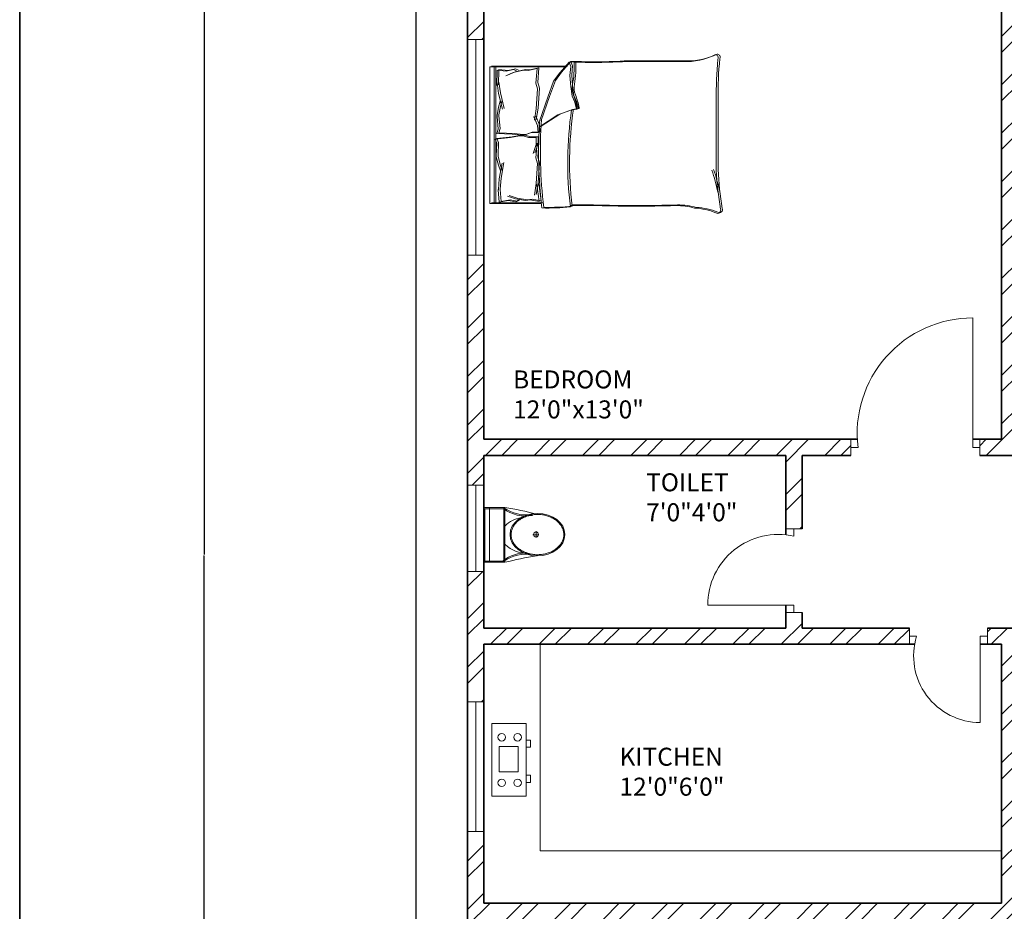
# Model space of a CAD drawing. Units: inches. Extents: x 1962 to 2771, y 1245 to 2660.
# Tile 85 of 114: x 1962 to 2236, y 2180 to 2428. Entities that reach past the tile are written whole.
import ezdxf

# ---------------------------------------------------------------- set-up
doc = ezdxf.new("R2010")
doc.units = ezdxf.units.IN
for name, color, linetype, lineweight in [('A-ANNO-DIMS', 2, 'Continuous', 18), ('A-ANNO-TTLB', 7, 'Continuous', 35), ('A-AREA-IDEN', 7, 'Continuous', 18), ('A-DOOR', 3, 'Continuous', 18), ('A-EQPM', 8, 'Continuous', 18), ('A-FLOR-CASE', 8, 'Continuous', 18), ('A-FLOR-FIXT', 8, 'Continuous', 18), ('A-FURN', 8, 'Continuous', 13), ('A-GLAZ', 4, 'Continuous', 18), ('A-WALL', 7, 'Continuous', 35), ('A-WALL-PATT', 252, 'Continuous', 13)]:
    doc.layers.add(name, color=color, linetype=linetype, lineweight=lineweight)
doc.styles.get("Standard").update_dxf_attribs({"font": 'arial.ttf'})
doc.dimstyles.get("Standard").update_dxf_attribs({"dimtxt": 0.18, "dimasz": 0.18, "dimexe": 0.18, "dimexo": 0.0625, "dimgap": 0.09, "dimtad": 0, "dimtih": 1, "dimtoh": 1, "dimdec": 4, "dimzin": 0, "dimdsep": 46, "dimtxsty": 'Standard', "dimcen": 0.09, "dimadec": 0, "dimazin": 0, "dimtfac": 1, "dimtdec": 4, "dimtofl": 0, "dimtmove": 0, "dimatfit": 3, "dimfxl": 1, "dimtolj": 1, "dimtzin": 0, "dimarcsym": 0})

# ---------------------------------------------------------------- blocks, each defined once
blk = doc.blocks.new('A$C31115884')
for p, q in [((283.1, 497.7), (223.4, 497.7)), ((257.5, 466.4), (257.5, 523.2)), ((0, 200), (0, 0)), ((520, 200), (0, 200)), ((10, 190), (10, 10)), ((510, 190), (10, 190)), ((510, 10), (510, 190)), ((520, 0), (520, 200)), ((510, 54.5), (0, 54.5)), ((10, 10), (510, 10)), ((0, 0), (520, 0))]:
    blk.add_line(p, q)
blk.add_circle((255.6, 496.4), 23.6)
for centre, radius, start, end in [((2777.7, -204.6), 2807, 165.4549, 171.71327), ((3237, 905), 2807, 188.28673, 194.5451), ((-294.5, 403.3), 364.7, 324.20913, 9.34987), ((-294.5, 403.3), 374.7, 324.20913, 9.34987), ((139.5, 406.2), 293.5, 315.84364, 2.65635), ((805.8, 403.3), 374.7, 179.20365, 215.79087), ((805.8, 403.3), 364.7, 170.65013, 215.79087), ((383.6, 406.2), 293.5, 190.27735, 224.15636)]:
    blk.add_arc(centre, radius, start, end)
blk.add_ellipse((256.2, 509.9), major_axis=(0, -260.7), ratio=0.772727)
blk.add_open_spline([(256.2, 259.2), (263.1, 259.2), (270, 259.7), (287.8, 262.3), (298.7, 265.1), (319.9, 273.1), (330.2, 278.4), (350.1, 291.1), (359.7, 298.7), (377.7, 315.9), (386.2, 325.5), (401.7, 346.6), (408.8, 358.1), (421.3, 382.5), (426.8, 395.5), (435.9, 422.4), (439.5, 436.4), (444.8, 465.1), (446.5, 479.7), (447.9, 509.2), (447.6, 524), (445, 553.3), (442.7, 567.8), (436.3, 596), (432.1, 609.7), (421.9, 636), (416, 648.6), (402.5, 672.1), (395, 683), (378.6, 703), (369.8, 712.1), (351.1, 728), (341.3, 734.8), (320.9, 746.2), (310.4, 750.7), (288.9, 757.3), (278, 759.4), (256, 761), (245, 760.6), (223.1, 757.2), (212.3, 754.3), (191.1, 746.1), (180.8, 740.7), (160.9, 727.8), (151.4, 720.1), (133.5, 702.7), (125.1, 693), (109.6, 671.7), (102.6, 660.2), (90.2, 635.7), (84.9, 622.7), (76, 595.6), (72.4, 581.6), (67.2, 552.9), (65.6, 538.2), (64.4, 508.8), (64.8, 494), (67.5, 464.7), (69.9, 450.2), (76.6, 422), (80.8, 408.3), (91.1, 382.2), (97.2, 369.7), (110.8, 346.3), (118.4, 335.4), (134.8, 315.6), (143.7, 306.7), (162.4, 290.9), (172.3, 284.2), (192.8, 273), (203.3, 268.6), (224.8, 262.2), (235.8, 260.2), (249.9, 259.3), (253, 259.2), (256.2, 259.2)], degree=3, knots=[0, 0, 0, 0, 0.110105, 0.110105, 0.285049, 0.285049, 0.459994, 0.459994, 0.634938, 0.634938, 0.809882, 0.809882, 0.984827, 0.984827, 1.159771, 1.159771, 1.334715, 1.334715, 1.50966, 1.50966, 1.684604, 1.684604, 1.859549, 1.859549, 2.034493, 2.034493, 2.209437, 2.209437, 2.384382, 2.384382, 2.559326, 2.559326, 2.73427, 2.73427, 2.909215, 2.909215, 3.084159, 3.084159, 3.259103, 3.259103, 3.434048, 3.434048, 3.608992, 3.608992, 3.783936, 3.783936, 3.958881, 3.958881, 4.133825, 4.133825, 4.30877, 4.30877, 4.483714, 4.483714, 4.658658, 4.658658, 4.833603, 4.833603, 5.008547, 5.008547, 5.183491, 5.183491, 5.358436, 5.358436, 5.53338, 5.53338, 5.708324, 5.708324, 5.883269, 5.883269, 6.058213, 6.058213, 6.233158, 6.233158, 6.283185, 6.283185, 6.283185, 6.283185])
blk = doc.blocks.new('BED-PLAN')
for p, q in [((22.05, 42.03), (19.47, 39.08)), ((22.05, 42.02), (19.47, 39.08)), ((22.56, 42.21), (19.98, 39.26)), ((22.56, 42.21), (19.98, 39.26)), ((23.44, 42.09), (22.05, 42.03, 3.08)), ((23.44, 42.09), (22.05, 42.02, 3.08)), ((22.55, 40.8), (22.05, 42.03)), ((22.55, 40.8), (22.05, 42.02)), ((23.95, 42.27), (22.56, 42.21, 3.08)), ((23.95, 42.27), (22.56, 42.21, 3.08)), ((23.06, 40.98), (22.56, 42.21)), ((23.06, 40.98), (22.56, 42.21)), ((0, 40.75), (21.15, 40.75)), ((0, 40.75), (21.15, 40.75)), ((0, 2.76), (0, 40.75)), ((0.51, 40.93), (21.66, 40.93)), ((0.51, 40.93), (21.66, 40.93)), ((1.22, 2.76), (1.22, 40.75)), ((1.22, 2.76), (1.22, 40.75)), ((1.73, 2.95), (1.73, 40.93)), ((1.73, 2.95), (1.73, 40.93)), ((2.03, 39.83), (1.96, 35.54)), ((2.03, 39.83), (1.96, 35.54)), ((2.03, 39.83), (4.58, 39.53)), ((2.03, 39.83), (4.58, 39.53)), ((2.54, 40.02), (2.46, 35.72)), ((2.54, 40.02), (2.46, 35.72)), ((2.54, 40.02), (5.09, 39.72)), ((2.54, 40.02), (5.09, 39.72)), ((6.56, 39.2), (4.43, 38.26)), ((6.56, 39.2), (4.43, 38.26)), ((4.58, 39.53), (6.63, 40.01)), ((4.58, 39.53), (6.63, 40.01)), ((7.07, 39.38), (4.94, 38.44)), ((7.07, 39.38), (4.94, 38.44)), ((5.09, 39.72), (7.14, 40.19)), ((5.09, 39.72), (7.14, 40.19)), ((9.4, 39.83), (6.56, 39.2)), ((9.4, 39.83), (6.56, 39.2)), ((6.63, 40.01), (7.46, 39.6)), ((6.63, 40.01), (7.46, 39.6)), ((9.91, 40.02), (7.07, 39.38)), ((9.91, 40.02), (7.07, 39.38)), ((7.14, 40.19), (7.97, 39.78)), ((7.14, 40.19), (7.97, 39.78)), ((10.68, 39.68), (9.4, 39.83)), ((10.68, 39.68), (9.4, 39.83)), ((11.19, 39.87), (9.91, 40.02)), ((11.19, 39.87), (9.91, 40.02)), ((13.17, 40.3), (10.68, 39.68)), ((13.17, 40.3), (10.68, 39.68)), ((13.68, 40.48), (11.19, 39.87)), ((13.68, 40.48), (11.19, 39.87)), ((12.85, 36.22), (13.17, 40.3)), ((12.85, 36.22), (13.17, 40.3)), ((13.36, 36.4), (13.68, 40.48)), ((13.36, 36.4), (13.68, 40.48)), ((19.47, 39.08), (17.75, 36.74)), ((19.47, 39.08), (17.75, 36.74)), ((19.98, 39.26), (18.26, 36.92)), ((19.98, 39.26), (18.26, 36.92)), ((22.3, 38.34), (22.55, 40.8)), ((22.3, 38.34), (22.55, 40.8)), ((22.55, 35.26), (22.3, 38.34)), ((22.55, 35.26), (22.3, 38.34)), ((22.81, 38.52), (23.06, 40.98)), ((22.81, 38.52), (23.06, 40.98)), ((23.06, 35.45), (22.81, 38.52)), ((23.06, 35.44), (22.81, 38.52)), ((1.96, 35.54), (2.02, 36.34)), ((1.96, 35.54), (2.02, 36.34)), ((2.02, 36.34), (2.44, 33.32)), ((2.02, 36.34), (2.44, 33.32)), ((2.46, 35.72), (2.53, 36.52)), ((2.46, 35.72), (2.53, 36.52)), ((2.53, 36.52), (2.95, 33.5)), ((2.53, 36.52), (2.95, 33.5)), ((13.3, 34.66), (12.85, 36.22)), ((13.3, 34.66), (12.85, 36.22)), ((13.8, 34.84), (13.36, 36.4)), ((13.8, 34.84), (13.36, 36.4)), ((17.75, 36.74), (16.15, 32.31)), ((17.75, 36.74), (16.15, 32.31)), ((18.26, 36.92), (16.66, 32.49)), ((18.26, 36.92), (16.66, 32.49)), ((2.44, 33.32), (3.52, 29.01)), ((2.44, 33.32), (3.52, 29.01)), ((2.95, 33.5), (4.02, 29.19)), ((2.95, 33.5), (4.02, 29.19)), ((12.95, 29.09), (13.3, 34.66)), ((12.95, 29.09), (13.3, 34.66)), ((13.46, 29.27), (13.8, 34.84)), ((13.46, 29.27), (13.8, 34.84)), ((22.92, 32.56), (22.55, 35.26)), ((22.92, 32.55), (22.55, 35.26)), ((23.42, 32.74), (23.06, 35.45)), ((23.42, 32.74), (23.06, 35.44)), ((2.92, 31.16), (2.45, 29.52)), ((2.92, 31.16), (2.45, 29.52)), ((3.43, 31.34), (2.96, 29.7)), ((3.43, 31.34), (2.96, 29.7)), ((16.15, 32.31), (13.82, 25.68)), ((16.15, 32.31), (13.82, 25.68)), ((16.66, 32.49), (14.33, 25.86)), ((16.66, 32.49), (14.33, 25.86)), ((23.65, 30.95), (22.92, 32.56)), ((23.65, 30.95), (22.92, 32.55)), ((24.16, 31.14), (23.42, 32.74)), ((24.16, 31.14), (23.42, 32.74)), ((24.15, 28.99), (23.65, 30.95)), ((24.15, 28.98), (23.65, 30.95)), ((24.65, 29.17), (24.16, 31.14)), ((24.65, 29.17), (24.16, 31.14)), ((62.99, 11.98), (62.99, 31.54)), ((62.99, 11.97), (62.99, 31.54)), ((63.5, 12.16), (63.5, 31.72)), ((63.5, 12.16), (63.5, 31.72)), ((2.45, 29.52), (2.02, 27.19)), ((2.45, 29.52), (2.02, 27.19)), ((2.96, 29.7), (2.52, 27.37)), ((2.96, 29.7), (2.52, 27.37)), ((12.42, 25.89), (12.95, 29.09)), ((12.42, 25.89), (12.95, 29.09)), ((12.93, 26.07), (13.46, 29.27)), ((12.93, 26.07), (13.46, 29.27)), ((13.82, 24.05), (18.98, 27.38)), ((13.82, 24.05), (18.98, 27.38)), ((14.33, 24.24), (19.49, 27.57)), ((14.33, 24.24), (19.49, 27.57)), ((18.98, 27.38), (22.55, 28.74)), ((18.98, 27.38), (22.55, 28.74)), ((19.49, 27.57), (23.06, 28.92)), ((19.49, 27.57), (23.06, 28.92)), ((22.55, 28.74), (24.15, 28.99)), ((22.55, 28.74), (24.15, 28.98)), ((23.06, 28.92), (24.65, 29.17)), ((23.06, 28.92), (24.65, 29.17)), ((2.02, 27.19), (2.03, 26.94)), ((2.02, 27.19), (2.03, 26.93)), ((2.03, 26.94), (2.37, 23.42)), ((2.03, 26.93), (2.37, 23.42)), ((2.52, 27.37), (2.54, 27.12)), ((2.52, 27.37), (2.54, 27.12)), ((2.54, 27.12), (2.88, 23.6)), ((2.54, 27.12), (2.88, 23.6)), ((13.31, 24.44), (12.28, 26.89)), ((13.31, 24.44), (12.28, 26.88)), ((13.81, 24.63), (12.79, 27.07)), ((13.81, 24.63), (12.79, 27.07)), ((2.37, 23.42), (1.98, 22.24)), ((2.37, 23.42), (1.98, 22.24)), ((1.98, 22.24), (6.25, 22.05)), ((1.98, 22.24), (6.25, 22.05)), ((2.88, 23.6), (2.49, 22.42)), ((2.88, 23.6), (2.49, 22.42)), ((2.49, 22.42), (6.76, 22.23)), ((2.49, 22.42), (6.76, 22.23)), ((6.25, 22.05), (8.81, 21.75)), ((6.25, 22.05), (8.81, 21.75)), ((6.76, 22.23), (9.31, 21.93)), ((6.76, 22.23), (9.31, 21.93)), ((9.31, 21.93), (10.35, 21.99)), ((9.31, 21.93), (10.35, 21.99)), ((9.84, 21.81), (11.3, 22.36)), ((9.84, 21.81), (11.3, 22.36)), ((10.35, 21.99), (11.81, 22.54)), ((10.35, 21.99), (11.81, 22.54)), ((11.3, 22.36), (13.43, 22.49)), ((11.3, 22.36), (13.43, 22.49)), ((11.81, 22.54), (13.94, 22.68)), ((11.81, 22.54), (13.94, 22.68)), ((13.43, 22.49), (13.31, 24.44)), ((13.43, 22.49), (13.31, 24.44)), ((13.94, 22.68), (13.81, 24.63)), ((13.94, 22.68), (13.81, 24.63)), ((1.49, 20.65), (5.74, 21.11)), ((1.49, 20.65), (5.74, 21.11)), ((1.95, 19.51), (1.49, 20.65)), ((1.95, 19.51), (1.49, 20.65)), ((1.83, 15.97), (1.95, 19.51)), ((1.83, 15.97), (1.95, 19.51)), ((1.99, 20.84), (6.25, 21.3)), ((1.99, 20.84), (6.25, 21.3)), ((2.45, 19.69), (1.99, 20.84)), ((2.45, 19.69), (1.99, 20.84)), ((2.34, 16.15), (2.45, 19.69)), ((2.34, 16.15), (2.45, 19.69)), ((5.74, 21.11), (8.27, 21.57)), ((5.74, 21.11), (8.27, 21.57)), ((6.25, 21.3), (8.78, 21.76)), ((6.25, 21.3), (8.78, 21.76)), ((8.27, 21.57), (9.3, 21.57)), ((8.27, 21.57), (9.3, 21.57)), ((8.78, 21.76), (9.81, 21.76)), ((8.78, 21.76), (9.81, 21.76)), ((8.81, 21.75), (9.84, 21.81)), ((8.81, 21.75), (9.84, 21.81)), ((9.3, 21.57), (10.8, 21.11)), ((9.3, 21.57), (10.8, 21.11)), ((9.81, 21.76), (11.3, 21.3)), ((9.81, 21.76), (11.3, 21.3)), ((10.8, 21.11), (12.93, 21.11)), ((10.8, 21.11), (12.93, 21.11)), ((11.3, 21.3), (13.44, 21.3)), ((11.3, 21.3), (13.44, 21.3)), ((13.44, 19.34), (12.57, 16.84)), ((13.44, 19.34), (12.57, 16.84)), ((12.85, 15.41), (13.17, 19.49)), ((12.85, 15.41), (13.17, 19.49)), ((12.93, 21.11), (12.93, 19.16)), ((12.93, 21.11), (12.93, 19.16)), ((13.36, 15.59), (13.68, 19.67)), ((13.36, 15.59), (13.68, 19.67)), ((13.44, 21.3), (13.44, 19.34)), ((13.44, 21.3), (13.44, 19.34)), ((12.93, 19.16), (12.06, 16.66)), ((12.93, 19.16), (12.06, 16.66)), ((1.83, 15.72), (1.83, 15.97)), ((1.83, 15.72), (1.83, 15.97)), ((2.41, 13.42), (1.83, 15.72)), ((2.41, 13.42), (1.83, 15.72)), ((2.34, 15.9), (2.34, 16.15)), ((2.34, 15.9), (2.34, 16.15)), ((2.91, 13.6), (2.34, 15.9)), ((2.91, 13.6), (2.34, 15.9)), ((2.64, 9.63), (3.44, 13.99)), ((2.64, 9.63), (3.44, 13.99)), ((3.14, 9.81), (3.95, 14.17)), ((3.14, 9.81), (3.95, 14.17)), ((13.3, 13.85), (12.85, 15.41)), ((13.3, 13.85), (12.85, 15.41)), ((12.95, 8.28), (13.3, 13.85)), ((12.95, 8.28), (13.3, 13.85)), ((13.8, 14.03), (13.36, 15.59)), ((13.8, 14.03), (13.36, 15.59)), ((13.46, 8.46), (13.8, 14.03)), ((13.46, 8.46), (13.8, 14.03)), ((2.98, 11.81), (2.41, 13.42)), ((2.98, 11.81), (2.41, 13.42)), ((3.49, 11.99), (2.91, 13.6)), ((3.49, 11.99), (2.91, 13.6)), ((2.41, 6.59), (2.64, 9.63)), ((2.41, 6.59), (2.64, 9.63)), ((2.91, 6.77), (3.14, 9.81)), ((2.91, 6.77), (3.14, 9.81)), ((12.42, 5.07), (12.95, 8.28)), ((12.42, 5.07), (12.95, 8.28)), ((12.93, 5.26), (13.46, 8.46)), ((12.93, 5.26), (13.46, 8.46)), ((12.95, 8.28), (13.21, 7.38)), ((12.95, 8.28), (13.21, 7.38)), ((13.46, 8.46), (13.72, 7.56)), ((13.46, 8.46), (13.72, 7.56)), ((2.39, 6.5), (2.41, 6.59)), ((2.39, 6.5), (2.41, 6.59)), ((2.65, 3.1), (2.39, 6.5)), ((2.65, 3.1), (2.39, 6.5)), ((2.9, 6.68), (2.91, 6.77)), ((2.9, 6.68), (2.91, 6.77)), ((3.16, 3.28), (2.9, 6.68)), ((3.16, 3.28), (2.9, 6.68)), ((13.21, 7.38), (13.78, 3.33)), ((13.21, 7.38), (13.78, 3.33)), ((13.72, 7.56), (14.29, 3.51)), ((13.72, 7.56), (14.29, 3.51)), ((14.4, 2.76), (0, 2.76)), ((14.4, 2.76), (0, 2.76)), ((14.9, 2.95), (0.51, 2.95)), ((14.9, 2.95), (0.51, 2.95)), ((2.64, 3.1), (5.16, 3.56)), ((2.64, 3.1), (5.16, 3.56)), ((3.14, 3.28), (5.67, 3.74)), ((3.14, 3.28), (5.67, 3.74)), ((7.12, 4.02), (4.93, 4.82)), ((7.12, 4.02), (4.93, 4.82)), ((5.16, 3.56), (7.23, 3.21)), ((5.16, 3.56), (7.23, 3.21)), ((7.63, 4.2), (5.44, 5)), ((7.63, 4.2), (5.44, 5)), ((5.67, 3.74), (7.74, 3.39)), ((5.67, 3.74), (7.74, 3.39)), ((9.99, 3.56), (7.12, 4.02)), ((9.99, 3.56), (7.12, 4.02)), ((7.23, 3.21), (8.04, 3.67)), ((7.23, 3.21), (8.04, 3.67)), ((10.5, 3.74), (7.63, 4.2)), ((10.5, 3.74), (7.63, 4.2)), ((7.74, 3.39), (8.55, 3.85)), ((7.74, 3.39), (8.55, 3.85)), ((11.26, 3.79), (9.99, 3.56)), ((11.26, 3.79), (9.99, 3.56)), ((11.76, 3.97), (10.5, 3.74)), ((11.76, 3.97), (10.5, 3.74)), ((13.78, 3.33), (11.26, 3.79)), ((13.78, 3.33), (11.26, 3.79)), ((14.29, 3.51), (11.76, 3.97)), ((14.29, 3.51), (11.76, 3.97))]:
    blk.add_line(p, q)
for centre, radius, start, end in [((54.58, 60.54), 18.33, 267.4714, 296.4681), ((54.58, 60.54), 18.33, 267.4714, 296.4681), ((55.09, 60.72), 18.33, 267.4714, 296.4681), ((55.09, 60.72), 18.33, 267.4714, 296.4681), ((62.69, 43.25), 0.876, 332.6588, 86.02), ((62.69, 43.25), 0.876, 332.6588, 86.02), ((63.2, 43.43), 0.876, 332.6588, 86.02), ((63.2, 43.43), 0.876, 332.6588, 86.02), ((-5.29, 40.8), 28.76, 349.8763, 2.5657), ((-5.29, 40.8), 28.76, 349.8763, 2.5657), ((28.87, 144.88), 102.94, 266.9791, 273.8365), ((28.87, 144.88), 102.94, 266.9791, 273.8365), ((-4.78, 40.98), 28.76, 349.8763, 2.5657), ((-4.78, 40.98), 28.76, 349.8763, 2.5657), ((29.37, 145.06), 102.94, 266.9791, 273.8365), ((29.37, 145.06), 102.94, 266.9791, 273.8365), ((53.91, -3583.94), 3626.16, 90.00217, 90.28689), ((53.91, -3583.94), 3626.16, 90.00217, 90.28689), ((54.42, -3583.75), 3626.16, 90.00217, 90.28689), ((54.42, -3583.75), 3626.16, 90.00217, 90.28689), ((168.74, 32.71), 105.75, 174.4998, 180.6351), ((168.74, 32.71), 105.75, 174.4998, 180.6351), ((169.24, 32.89), 105.75, 174.4998, 180.6351), ((169.24, 32.89), 105.75, 174.4998, 180.6351), ((27.87, 34.77), 4.95, 168.6608, 203.7384), ((27.87, 34.77), 4.95, 168.6608, 203.7384), ((28.38, 34.95), 4.95, 168.6608, 203.7384), ((28.38, 34.95), 4.95, 168.6608, 203.7384), ((1.69, 24.95), 23.57, 10.6617, 19.8806), ((1.69, 24.95), 23.57, 10.6617, 19.8806), ((1.18, 24.77), 23.57, 10.6617, 19.8806), ((1.18, 24.76), 23.57, 10.6617, 19.8806), ((124.25, 14.12), 102.56, 171.7845, 186.9006), ((124.25, 14.11), 102.56, 171.7845, 186.9006), ((124.76, 14.3), 102.56, 171.7845, 186.9006), ((124.76, 14.3), 102.56, 171.7845, 186.9006), ((24.2, 29.12), 0.147, 250.2464, 1.1377), ((24.2, 29.12), 0.147, 250.2464, 1.1377), ((24.7, 29.3), 0.147, 250.2464, 1.1377), ((24.7, 29.3), 0.147, 250.2464, 1.1377), ((144.71, 16.98), 131.13, 176.0865, 186.7821), ((144.71, 16.98), 131.13, 176.0865, 186.7821), ((145.22, 17.16), 131.13, 176.0865, 186.7821), ((145.22, 17.16), 131.13, 176.0865, 186.7821), ((-18.85, -13.69), 84.62, 13.3832, 17.7053), ((-18.85, -13.69), 84.62, 13.3832, 17.7053), ((-18.34, -13.51), 84.62, 13.3832, 17.7053), ((-18.34, -13.51), 84.62, 13.3832, 17.7053), ((159.64, 17.03), 96.78, 182.9958, 189.4091), ((159.64, 17.03), 96.78, 182.9958, 189.4091), ((160.15, 17.21), 96.78, 182.9958, 189.4091), ((160.15, 17.21), 96.78, 182.9958, 189.4091), ((15.97, 67.7), 66.22, 268.7218, 275.604), ((15.97, 67.7), 66.22, 268.7218, 275.604), ((16.48, 67.88), 66.22, 268.7218, 275.604), ((16.48, 67.88), 66.22, 268.7218, 275.604), ((24.78, -132.99), 135.22, 88.4762, 91.0082), ((24.78, -132.99), 135.22, 88.4762, 91.0082), ((25.29, -132.81), 135.22, 88.4762, 91.0082), ((25.29, -132.81), 135.22, 88.4762, 91.0082), ((40.23, 385.38), 383.38, 268.2277, 271.7185), ((40.23, 385.38), 383.38, 268.2277, 271.7185), ((40.74, 385.56), 383.38, 268.2277, 271.7185), ((40.74, 385.56), 383.38, 268.2277, 271.7185), ((51.28, -21.38), 23.56, 76.0648, 88.9113), ((51.28, -21.38), 23.56, 76.0648, 88.9113), ((51.79, -21.2), 23.56, 76.0648, 88.9113), ((51.79, -21.2), 23.56, 76.0648, 88.9113), ((55.86, -17.22), 18.73, 67.9751, 86.652), ((55.86, -17.22), 18.73, 67.9751, 86.652), ((56.37, -17.03), 18.73, 67.9751, 86.652), ((56.37, -17.03), 18.73, 67.9751, 86.652), ((63.37, 0.87), 0.866, 236.1736, 23.4781), ((63.37, 0.87), 0.866, 236.1736, 23.4781), ((63.87, 1.05), 0.866, 236.1736, 23.4781), ((63.87, 1.05), 0.866, 236.1736, 23.4781)]:
    blk.add_arc(centre, radius, start, end)
blk = doc.blocks.new('COOKTOP-4-BURNER')
for points in [[(0, 20.18), (9.48, 20.18), (9.48, 0), (0, 0)], [(2, 13.79), (7.26, 13.79), (7.26, 6.73), (2, 6.73)], [(9.48, 15.59), (10.71, 15.59), (10.71, 13.59), (9.48, 13.59)], [(9.48, 5.81), (10.71, 5.81), (10.71, 3.8), (9.48, 3.8)]]:
    blk.add_lwpolyline(points, close=True)
for centre in [(2.74, 16.38), (7.14, 16.38), (2.74, 3.71), (7.14, 3.71)]:
    blk.add_circle(centre, 1.05)
blk = doc.blocks.new('WIN-24IN-A')
for p, q in [((0, 24), (4.5, 24)), ((4.5, 24), (2.25, 24)), ((2.25, 24), (2.25, 0)), ((2.25, 0), (0, 0)), ((0, 0), (4.5, 0))]:
    blk.add_line(p, q)
blk = doc.blocks.new('WIN-60IN-A')
for p, q in [((0, 60), (4.5, 60)), ((4.5, 60), (2.25, 60)), ((2.25, 60), (2.25, 0)), ((2.25, 0), (0, 0)), ((0, 0), (4.5, 0))]:
    blk.add_line(p, q)
blk = doc.blocks.new('WIN-36IN-A')
for p, q in [((4.5, 36), (0, 36)), ((0, 36), (2.25, 36)), ((2.25, 36), (2.25, 0)), ((2.25, 0), (0, 0)), ((0, 0), (4.5, 0))]:
    blk.add_line(p, q)
blk = doc.blocks.new('*D40')
at = {"layer": 'A-ANNO-DIMS', "color": 0, "lineweight": -2, "transparency": 16777216}
for p, q in [((2072.02, 2033.91), (2072.02, 2583.47)), ((2072.2, 2583.29), (2366.02, 2583.29)), ((2660.63, 2583.29), (2366.81, 2583.29)), ((2660.81, 2524.41), (2660.81, 2583.47))]:
    blk.add_line(p, q, dxfattribs=at)
at = {"layer": 'A-ANNO-DIMS', "color": 0, "transparency": 16777216}
for points in [[(2072.2, 2583.32), (2072.2, 2583.26), (2072.02, 2583.29)], [(2660.63, 2583.32), (2660.63, 2583.26), (2660.81, 2583.29)]]:
    blk.add_solid(points, dxfattribs=at)
at = {"layer": 'Defpoints', "color": 0, "transparency": 16777216}
for p in [(2660.81, 2583.29), (2660.81, 2524.34), (2072.02, 2033.84)]:
    blk.add_point(p, dxfattribs=at)
at = {"layer": 'A-ANNO-DIMS', "color": 0, "transparency": 16777216, "insert": (2366.41, 2583.29), "char_height": 0.18, "attachment_point": 5}
blk.add_mtext('\\A1;588.8', dxfattribs=at)
blk = doc.blocks.new('*D43')
at = {"layer": 'A-ANNO-DIMS', "color": 0, "lineweight": -2, "transparency": 16777216}
for p, q in [((2086.24, 2524.34), (2012.89, 2524.34)), ((2013.07, 2524.16), (2013.07, 2279.28)), ((2013.07, 2034.02), (2013.07, 2278.91)), ((2071.96, 2033.84), (2012.89, 2033.84))]:
    blk.add_line(p, q, dxfattribs=at)
at = {"layer": 'A-ANNO-DIMS', "color": 0, "transparency": 16777216}
for points in [[(2013.04, 2524.16), (2013.1, 2524.16), (2013.07, 2524.34)], [(2013.04, 2034.02), (2013.1, 2034.02), (2013.07, 2033.84)]]:
    blk.add_solid(points, dxfattribs=at)
at = {"layer": 'Defpoints', "color": 0, "transparency": 16777216}
for p in [(2086.31, 2524.34), (2013.07, 2033.84), (2072.02, 2033.84)]:
    blk.add_point(p, dxfattribs=at)
at = {"layer": 'A-ANNO-DIMS', "color": 0, "transparency": 16777216, "insert": (2013.07, 2279.09), "char_height": 0.18, "attachment_point": 5}
blk.add_mtext('\\A1;490.5', dxfattribs=at)

msp = doc.modelspace()

# ---------------------------------------------------------------- hatches: boundary and pattern name
at = {"layer": 'A-WALL-PATT'}
h = msp.add_hatch(dxfattribs=at)
h.set_pattern_fill('ANSI32', color=256)
h.paths.add_polyline_path([(2090.8074, 2467.3437), (2141.6481, 2467.3437), (2141.6481, 2469.5937), (2141.6481, 2471.8437), (2086.3074, 2471.8437), (2086.3074, 2422.5333), (2090.8074, 2422.5333)])
h.paths.add_polyline_path([(2282.7664, 2471.8437), (2204.8982, 2471.8437), (2204.8982, 2467.3437), (2234.8074, 2467.3437), (2234.8074, 2311.3437), (2228.7492, 2311.3437), (2228.7492, 2306.8437), (2234.8074, 2306.8437), (2331.9227, 2306.8437), (2331.9227, 2309.0937), (2331.9227, 2311.3437), (2239.3074, 2311.3437), (2239.3074, 2467.3437), (2282.7664, 2467.3437), (2282.7664, 2469.5937)])
h.paths.add_polyline_path([(2471.4531, 2519.8437), (2552.011, 2519.8437), (2564.3996, 2519.8437), (2564.3996, 2511.1389), (2568.8996, 2511.1389), (2568.8996, 2524.3437), (2466.9531, 2524.3437), (2466.9531, 2471.8437), (2450.0749, 2471.8437), (2446.4672, 2471.8437), (2446.4672, 2467.3437), (2450.0749, 2467.3437), (2475.9988, 2467.3437), (2475.9988, 2469.5937), (2475.9988, 2471.8437), (2471.4531, 2471.8437)])
h.paths.add_polyline_path([(2575.2231, 2469.5937), (2575.2231, 2471.8437), (2568.8996, 2471.8437), (2568.8996, 2487.1389), (2564.3996, 2487.1389), (2564.3996, 2471.8437), (2556.511, 2471.8437), (2499.2904, 2471.8437), (2499.2904, 2467.3437), (2507.8074, 2467.3437), (2507.8074, 2311.3437), (2414.863, 2311.3437), (2414.863, 2306.8437), (2512.3074, 2306.8437), (2517.0114, 2306.8437), (2517.0114, 2309.0937), (2517.0114, 2311.3437), (2512.3074, 2311.3437), (2512.3074, 2467.3437), (2575.2231, 2467.3437)])
h.paths.add_polyline_path([(2660.8074, 2471.8437), (2600.9602, 2471.8437), (2600.9602, 2467.3437), (2656.3074, 2467.3437), (2656.3074, 2432.5704), (2660.8074, 2432.5704)])
h.paths.add_polyline_path([(2660.8074, 2372.5704), (2656.3074, 2372.5704), (2656.3074, 2311.3437), (2600.276, 2311.3437), (2600.276, 2309.0937), (2600.276, 2306.8437), (2656.3074, 2306.8437), (2656.3074, 2296.2593), (2660.8074, 2296.2593)])
h.paths.add_polyline_path([(2572.3074, 2306.8437), (2577.1385, 2306.8437), (2577.1385, 2311.3437), (2551.082, 2311.3437), (2551.082, 2306.8437), (2567.8074, 2306.8437), (2567.8074, 2258.8437), (2540.0574, 2258.8437), (2540.0574, 2256.5937), (2540.0574, 2254.3437), (2567.8074, 2254.3437), (2656.3074, 2254.3437), (2656.3074, 2236.9085), (2660.8074, 2236.9085), (2660.8074, 2272.2593), (2656.3074, 2272.2593), (2656.3074, 2258.8437), (2572.3074, 2258.8437)])
h.paths.add_polyline_path([(2512.3074, 2254.3437), (2518.8716, 2254.3437), (2518.8716, 2256.5937), (2518.8716, 2258.8437), (2507.8074, 2258.8437), (2507.8074, 2177.8437), (2567.8074, 2177.8437), (2567.8074, 2172.9628), (2572.3074, 2172.9628), (2572.3074, 2177.8437), (2656.3074, 2177.8437), (2656.3074, 2166.4846), (2660.8074, 2166.4846), (2660.8074, 2200.9085), (2656.3074, 2200.9085), (2656.3074, 2182.3437), (2512.3074, 2182.3437)])
h.paths.add_polyline_path([(2656.3074, 2129.8437), (2572.3074, 2129.8437), (2572.3074, 2150.3044), (2570.0574, 2150.3044), (2567.8074, 2150.3044), (2567.8074, 2129.8437), (2507.8074, 2129.8437), (2507.8074, 2116.3027), (2510.0574, 2116.3027), (2512.3074, 2116.3027), (2512.3074, 2125.3437), (2567.8074, 2125.3437), (2572.3074, 2125.3437), (2656.3074, 2125.3437)])
h.paths.add_polyline_path([(2090.8074, 2362.5333), (2086.3074, 2362.5333), (2086.3074, 2298.6242), (2090.8074, 2298.6242), (2090.8074, 2306.8437), (2174.8074, 2306.8437), (2174.8074, 2286.4178), (2179.3074, 2286.4178), (2179.3074, 2306.8437), (2192.8641, 2306.8437), (2192.8641, 2309.0937), (2192.8641, 2311.3437), (2090.8074, 2311.3437)])
h.paths.add_polyline_path([(2209.156, 2258.8437), (2179.3074, 2258.8437), (2179.3074, 2263.2236), (2177.0574, 2263.2236), (2174.8074, 2263.2236), (2174.8074, 2258.8437), (2090.8074, 2258.8437), (2090.8074, 2274.6242), (2086.3074, 2274.6242), (2086.3074, 2238.2967), (2088.5574, 2238.2967), (2090.8074, 2238.2967), (2090.8074, 2254.3437), (2209.156, 2254.3437)])
h.paths.add_polyline_path([(2090.8074, 2177.8437), (2234.8074, 2177.8437), (2234.8074, 2173.1428), (2239.3074, 2173.1428), (2239.3074, 2258.8437), (2230.8442, 2258.8437), (2230.8442, 2256.5937), (2230.8442, 2254.3437), (2234.8074, 2254.3437), (2234.8074, 2182.3437), (2090.8074, 2182.3437), (2090.8074, 2202.2967), (2086.3074, 2202.2967), (2086.3074, 2140.0389), (2090.8074, 2140.0389)])
h.paths.add_polyline_path([(2090.8074, 2080.0389), (2086.3074, 2080.0389), (2086.3074, 2033.8437), (2090.8074, 2033.8437)], flags=17)
h.paths.add_polyline_path([(2244.9405, 2033.8437), (2239.3074, 2033.8437), (2239.3074, 2142.0665), (2237.2592, 2142.0665), (2234.8074, 2142.0665), (2234.8074, 2033.8437), (2090.8074, 2033.8437), (2076.5204, 2033.8437), (2072.0204, 2033.8437), (2072.0204, 2000.4493), (2076.5204, 2000.4493), (2076.5204, 2029.3437), (2090.8074, 2029.3437), (2244.9405, 2029.3437), (2244.9405, 2031.5937)])
h.paths.add_polyline_path([(2234.8074, 1933.3437), (2076.5204, 1933.3437), (2076.5204, 1952.4493), (2074.2704, 1952.4493), (2072.0204, 1952.4493), (2072.0204, 1933.3437), (2072.0204, 1928.8437), (2234.8074, 1928.8437)])
h.paths.add_polyline_path([(2090.8074, 1928.8437), (2086.3074, 1928.8437), (2086.3074, 1906.5013), (2090.8074, 1906.5013)])
h.paths.add_polyline_path([(2090.8074, 1846.5013), (2086.3074, 1846.5013), (2086.3074, 1769.9917), (2088.5574, 1769.9917), (2090.8074, 1769.9917), (2090.8074, 1780.3437), (2234.8074, 1780.3437), (2234.8074, 1708.3437), (2230.3764, 1708.3437), (2230.3764, 1703.8437), (2239.3074, 1703.8437), (2239.3074, 1792.6669), (2237.0574, 1792.6669), (2234.8074, 1792.6669), (2234.8074, 1784.8437), (2090.8074, 1784.8437)])
h.paths.add_polyline_path([(2239.3074, 1928.8437), (2244.9405, 1928.8437), (2244.9405, 1931.0937), (2244.9405, 1933.3437), (2234.8074, 1933.3437), (2234.8074, 1928.8437), (2234.8074, 1825.5949), (2239.3074, 1825.5949)])
h.paths.add_polyline_path([(2148.0425, 1649.0937), (2148.0425, 1651.3437), (2090.8074, 1651.3437), (2090.8074, 1646.8437), (2148.0425, 1646.8437)], flags=0)
h.paths.add_polyline_path([(2207.5601, 1708.3437), (2090.8074, 1708.3437), (2090.8074, 1703.8437), (2174.8074, 1703.8437), (2174.8074, 1651.3437), (2170.4457, 1651.3437), (2170.4457, 1646.8437), (2195.9924, 1646.8437), (2195.9924, 1649.0937), (2195.9924, 1651.3437), (2179.3074, 1651.3437), (2179.3074, 1703.8437), (2207.5601, 1703.8437), (2207.5601, 1706.0937)])
h.paths.add_polyline_path([(2090.8074, 1733.9917), (2086.3074, 1733.9917), (2086.3074, 1696.1032), (2088.5574, 1696.1032), (2090.8074, 1696.1032)])
h.paths.add_polyline_path([(2090.8074, 1672.1032), (2086.3074, 1672.1032), (2086.3074, 1600.3335), (2090.8074, 1600.3335)])
h.paths.add_polyline_path([(2090.8074, 1540.3335), (2086.3074, 1540.3335), (2086.3074, 1486.3437), (2139.6766, 1486.3437), (2139.6766, 1490.8437), (2090.8074, 1490.8437)])
h.paths.add_polyline_path([(2302.3876, 1490.8437), (2239.3074, 1490.8437), (2239.3074, 1646.8437), (2335.9994, 1646.8437), (2335.9994, 1651.3437), (2229.884, 1651.3437), (2229.884, 1646.8437), (2234.8074, 1646.8437), (2234.8074, 1490.8437), (2202.7103, 1490.8437), (2202.7103, 1488.5937), (2202.7103, 1486.3437), (2275.0699, 1486.3437), (2275.0699, 1475.772), (2279.5699, 1475.772), (2279.5699, 1486.3437), (2302.3876, 1486.3437)])
h.paths.add_polyline_path([(2279.5699, 1451.772), (2275.0699, 1451.772), (2275.0699, 1438.3437), (2174.8074, 1438.3437), (2174.8074, 1486.3437), (2179.7922, 1486.3437), (2179.7922, 1490.8437), (2163.3585, 1490.8437), (2163.3585, 1488.5937), (2163.3585, 1486.3437), (2170.3074, 1486.3437), (2170.3074, 1433.8437), (2279.5699, 1433.8437)])
h.paths.add_polyline_path([(2427.2363, 1490.8437), (2375.8074, 1490.8437), (2375.8074, 1646.8437), (2381.6401, 1646.8437), (2381.6401, 1651.3437), (2365.887, 1651.3437), (2365.887, 1649.0937), (2365.887, 1646.8437), (2371.3074, 1646.8437), (2371.3074, 1490.8437), (2327.5627, 1490.8437), (2327.5627, 1488.5937), (2327.5627, 1486.3437), (2371.3074, 1486.3437), (2371.3074, 1433.8437), (2375.8074, 1433.8437), (2375.8074, 1486.3437), (2427.2363, 1486.3437)])
h.paths.add_polyline_path([(2512.3074, 1646.8437), (2519.4351, 1646.8437), (2519.4351, 1649.0937), (2519.4351, 1651.3437), (2507.8074, 1651.3437), (2416.0063, 1651.3437), (2416.0063, 1649.0937), (2416.0063, 1646.8437), (2507.8074, 1646.8437), (2507.8074, 1490.8437), (2497.0532, 1490.8437), (2497.0532, 1488.5937), (2497.0532, 1486.3437), (2574.9344, 1486.3437), (2574.9344, 1476.0181), (2579.4344, 1476.0181), (2579.4344, 1486.3437), (2584.4872, 1486.3437), (2584.3074, 1490.8437), (2512.3074, 1490.8437)])
h.paths.add_polyline_path([(2470.5091, 1486.3437), (2473.9767, 1486.3437), (2473.9767, 1490.8437), (2449.6605, 1490.8437), (2449.6605, 1488.5937), (2449.6605, 1486.3437), (2466.0091, 1486.3437), (2466.0091, 1433.8437), (2470.5091, 1433.8437), (2579.4344, 1433.8437), (2579.4344, 1452.0181), (2574.9344, 1452.0181), (2574.9344, 1438.3437), (2554.5091, 1438.3437), (2470.5091, 1438.3437)])
h.paths.add_polyline_path([(2656.3074, 1490.8437), (2611.86, 1490.8437), (2611.86, 1486.3437), (2656.3074, 1486.3437)])
h.paths.add_polyline_path([(2660.8074, 1532.7007), (2658.5574, 1532.7007), (2656.3074, 1532.7007), (2656.3074, 1486.3437), (2660.8074, 1486.3437)])
h.paths.add_polyline_path([(2660.8074, 1664.9663), (2656.3074, 1664.9663), (2656.3074, 1651.3437), (2602.2313, 1651.3437), (2602.2313, 1646.8437), (2656.3074, 1646.8437), (2656.3074, 1592.7007), (2660.8074, 1592.7007)])
h.paths.add_polyline_path([(2660.8074, 1724.5221), (2656.3074, 1724.5221), (2656.3074, 1703.8437), (2542.4725, 1703.8437), (2542.4725, 1699.3437), (2567.8074, 1699.3437), (2567.8074, 1651.3437), (2552.7766, 1651.3437), (2552.7766, 1649.0937), (2552.7766, 1646.8437), (2577.2878, 1646.8437), (2577.2878, 1649.0937), (2577.2878, 1651.3437), (2572.3074, 1651.3437), (2572.3074, 1699.3437), (2656.3074, 1699.3437), (2656.3074, 1688.9663), (2660.8074, 1688.9663)])
h.paths.add_polyline_path([(2660.8074, 1880.6524), (2656.3074, 1880.6524), (2656.3074, 1832.8437), (2512.3074, 1832.8437), (2512.3074, 1837.8959), (2507.8074, 1837.8959), (2507.8074, 1828.3437), (2567.8074, 1828.3437), (2567.8074, 1804.3437), (2572.3074, 1804.3437), (2572.3074, 1828.3437), (2656.3074, 1828.3437), (2656.3074, 1818.6778), (2660.8074, 1818.6778)])
h.paths.add_polyline_path([(2660.8074, 1794.6778), (2656.3074, 1794.6778), (2656.3074, 1780.3437), (2572.3074, 1780.3437), (2572.3074, 1783.0303), (2570.0574, 1783.0303), (2567.8074, 1783.0303), (2567.8074, 1780.3437), (2507.8074, 1780.3437), (2507.8074, 1699.3437), (2517.8858, 1699.3437), (2517.8858, 1701.5937), (2517.8858, 1703.8437), (2512.3074, 1703.8437), (2512.3074, 1775.8437), (2656.3074, 1775.8437), (2656.3074, 1760.5221), (2660.8074, 1760.5221)])
h.paths.add_polyline_path([(2660.8074, 1981.3437), (2660.8074, 2020.2808), (2658.5574, 2020.2808), (2656.3074, 2020.2808), (2656.3074, 1981.3437), (2512.3074, 1981.3437), (2512.3074, 2086.6996), (2507.8074, 2086.6996), (2507.8074, 1981.3437), (2375.8074, 1981.3437), (2375.8074, 1986.8505), (2373.5574, 1986.8505), (2371.3074, 1986.8505), (2371.3074, 1973.2607), (2375.8074, 1973.2607), (2375.8074, 1976.8437), (2507.8074, 1976.8437), (2507.8074, 1865.4281), (2510.0574, 1865.4281), (2512.3074, 1865.4281), (2512.3074, 1976.8437), (2660.8074, 1976.8437)])
h.paths.add_polyline_path([(2375.8074, 1940.297), (2373.5574, 1940.297), (2371.3074, 1940.297), (2371.3074, 1933.3437), (2278.4434, 1933.3437), (2278.4434, 1928.8437), (2371.3074, 1928.8437), (2371.3074, 1651.3437), (2375.8074, 1651.3437)])
h.paths.add_polyline_path([(2660.8074, 1976.8437), (2656.3074, 1976.8437), (2656.3074, 1940.6524), (2660.8074, 1940.6524)], flags=17)
h.paths.add_polyline_path([(2660.8074, 2142.4846), (2656.3074, 2142.4846), (2656.3074, 2080.2808), (2660.8074, 2080.2808)])
h.paths.add_polyline_path([(2381.4189, 2311.3437), (2375.8074, 2311.3437), (2375.8074, 2467.3437), (2424.7242, 2467.3437), (2424.7242, 2469.5937), (2424.7242, 2471.8437), (2375.8074, 2471.8437), (2375.8074, 2524.3437), (2371.3074, 2524.3437), (2371.3074, 2471.8437), (2307.2097, 2471.8437), (2307.2097, 2467.3437), (2371.3074, 2467.3437), (2371.3074, 2311.3437), (2366.8901, 2311.3437), (2366.8901, 2306.8437), (2371.3074, 2306.8437), (2371.3074, 2033.8437), (2279.6589, 2033.8437), (2279.6589, 2029.3437), (2371.3074, 2029.3437), (2371.3074, 2014.2598), (2375.8074, 2014.2598), (2375.8074, 2306.8437), (2381.4189, 2306.8437)])
h.paths.add_polyline_path([(2263.3074, 2524.3437), (2170.3074, 2524.3437), (2170.3074, 2519.8437), (2170.3074, 2471.8437), (2165.0312, 2471.8437), (2165.0312, 2467.3437), (2179.6721, 2467.3437), (2179.6721, 2469.5161), (2179.6721, 2471.8437), (2174.8074, 2471.8437), (2174.8074, 2519.8437), (2258.8074, 2519.8437), (2258.8074, 2511.6436), (2263.3074, 2511.6436)])
h.paths.add_polyline_path([(2245.0232, 1361.4123), (2492.9468, 1361.4123), (2492.9468, 1398.505), (2245.0232, 1398.505)], flags=9)
h.paths.add_polyline_path([(2388.1434, 2086.6936), (2425.0704, 2086.6936), (2425.0704, 2105.3509), (2388.1434, 2105.3509)], flags=9)
h.paths.add_polyline_path([(2404.922, 2242.6744), (2445.7337, 2242.6744), (2445.7337, 2261.3318), (2404.922, 2261.3318)], flags=9)
h.paths.add_polyline_path([(2269.4107, 2156.7935), (2306.3378, 2156.7935), (2306.3378, 2175.4508), (2269.4107, 2175.4508)], flags=9)
h.paths.add_polyline_path([(2269.3277, 2233.4343), (2306.2547, 2233.4343), (2306.2547, 2252.0917), (2269.3277, 2252.0917)], flags=9)
h.paths.add_polyline_path([(2431.6052, 2320.6922), (2470.4456, 2320.6922), (2470.4456, 2339.3495), (2431.6052, 2339.3495)], flags=25)
h.paths.add_polyline_path([(2249.6902, 2315.7608), (2288.5306, 2315.7608), (2288.5306, 2334.4182), (2249.6902, 2334.4182)], flags=25)
h.paths.add_polyline_path([(2096.9301, 2314.3181), (2135.7704, 2314.3181), (2135.7704, 2332.9755), (2096.9301, 2332.9755)], flags=25)
h.paths.add_polyline_path([(2134.3475, 2285.7089), (2161.4655, 2285.7089), (2161.4655, 2304.3662), (2134.3475, 2304.3662)], flags=9)
h.paths.add_polyline_path([(2126.5155, 2209.4076), (2159.9227, 2209.4076), (2159.9227, 2228.065), (2126.5155, 2228.065)], flags=25)
h.paths.add_polyline_path([(2110.5753, 2141.5299), (2149.4157, 2141.5299), (2149.4157, 2160.1872), (2110.5753, 2160.1872)], flags=25)
h.paths.add_polyline_path([(2249.8618, 1968.3317), (2286.3966, 1968.3317), (2286.3966, 1986.989), (2249.8618, 1986.989)], flags=9)
h.paths.add_polyline_path([(2395.9507, 1777.0051), (2436.7624, 1777.0051), (2436.7624, 1795.6625), (2395.9507, 1795.6625)], flags=9)
h.paths.add_polyline_path([(2398.5259, 1888.5651), (2435.0062, 1888.5651), (2435.0062, 1907.2224), (2398.5259, 1907.2224)], flags=25)
h.paths.add_polyline_path([(2259.3506, 1728.3559), (2296.2776, 1728.3559), (2296.2776, 1747.0132), (2259.3506, 1747.0132)], flags=9)
h.paths.add_polyline_path([(2271.3698, 1845.268), (2308.2968, 1845.268), (2308.2968, 1863.9253), (2271.3698, 1863.9253)], flags=9)
h.paths.add_polyline_path([(2120.9355, 1786.3027), (2159.7759, 1786.3027), (2159.7759, 1804.9601), (2120.9355, 1804.9601)], flags=25)
h.paths.add_polyline_path([(2121.3164, 1732.1043), (2154.7236, 1732.1043), (2154.7236, 1750.7616), (2121.3164, 1750.7616)], flags=25)
h.paths.add_polyline_path([(2118.3706, 1678.8997), (2147.5282, 1678.8997), (2147.5282, 1697.557), (2118.3706, 1697.557)], flags=25)
h.paths.add_polyline_path([(2385.9227, 1493.557), (2424.763, 1493.557), (2424.763, 1512.2143), (2385.9227, 1512.2143)], flags=25)
h.paths.add_polyline_path([(2248.7058, 1500.0256), (2287.5462, 1500.0256), (2287.5462, 1518.6829), (2248.7058, 1518.6829)], flags=25)
h.paths.add_polyline_path([(2104.1669, 1617.3771), (2143.0073, 1617.3771), (2143.0073, 1636.0344), (2104.1669, 1636.0344)], flags=9)
h.paths.add_polyline_path([(2096.0714, 1447.8824), (2137.3845, 1447.8824), (2137.3845, 1458.1859), (2096.0714, 1458.1859)], flags=9)
h.paths.add_polyline_path([(2180.6114, 1440.325), (2209.7689, 1440.325), (2209.7689, 1458.9823), (2180.6114, 1458.9823)], flags=25)
h.paths.add_polyline_path([(2316.1698, 1447.9637), (2357.4829, 1447.9637), (2357.4829, 1458.2673), (2316.1698, 1458.2673)], flags=9)
h.paths.add_polyline_path([(2397.6187, 1447.9637), (2438.9318, 1447.9637), (2438.9318, 1458.2673), (2397.6187, 1458.2673)], flags=9)
h.paths.add_polyline_path([(2473.0778, 1439.5953), (2502.2354, 1439.5953), (2502.2354, 1458.2527), (2473.0778, 1458.2527)], flags=25)
h.paths.add_polyline_path([(2589.7027, 1447.8819), (2631.0158, 1447.8819), (2631.0158, 1458.1855), (2589.7027, 1458.1855)], flags=9)
h.paths.add_polyline_path([(2522.4009, 1497.5285), (2561.2413, 1497.5285), (2561.2413, 1516.1859), (2522.4009, 1516.1859)], flags=25)
h.paths.add_polyline_path([(2579.6565, 1671.3482), (2608.8141, 1671.3482), (2608.8141, 1690.0056), (2579.6565, 1690.0056)], flags=25)
h.paths.add_polyline_path([(2544.7038, 1725.5064), (2578.1111, 1725.5064), (2578.1111, 1744.1637), (2544.7038, 1744.1637)], flags=25)
h.paths.add_polyline_path([(2578.1191, 1807.472), (2607.2766, 1807.472), (2607.2766, 1826.1293), (2578.1191, 1826.1293)], flags=25)
h.paths.add_polyline_path([(2595.0614, 1835.1839), (2633.9018, 1835.1839), (2633.9018, 1853.8413), (2595.0614, 1853.8413)], flags=25)
h.paths.add_polyline_path([(2567.0097, 2097.7035), (2605.8501, 2097.7035), (2605.8501, 2116.3609), (2567.0097, 2116.3609)], flags=9)
h.paths.add_polyline_path([(2586.644, 2134.6454), (2615.8015, 2134.6454), (2615.8015, 2153.3027), (2586.644, 2153.3027)], flags=9)
h.paths.add_polyline_path([(2544.6185, 2212.6783), (2578.0258, 2212.6783), (2578.0258, 2231.3356), (2544.6185, 2231.3356)], flags=25)
h.paths.add_polyline_path([(2577.0273, 2256.9023), (2606.1849, 2256.9023), (2606.1849, 2275.5597), (2577.0273, 2275.5597)], flags=24)
h.paths.add_polyline_path([(2605.2683, 2315.2821), (2644.1087, 2315.2821), (2644.1087, 2333.9395), (2605.2683, 2333.9395)], flags=25)
h.paths.add_polyline_path([(2583.1244, 2496.1815), (2624.4375, 2496.1815), (2624.4375, 2506.4851), (2583.1244, 2506.4851)], flags=9)
h.paths.add_polyline_path([(2474.761, 2497.0823), (2503.9185, 2497.0823), (2503.9185, 2515.7397), (2474.761, 2515.7397)], flags=25)
h.paths.add_polyline_path([(2387.5787, 2494.2563), (2428.902, 2494.2563), (2428.902, 2504.5598), (2387.5787, 2504.5598)], flags=9)
h.paths.add_polyline_path([(2300.1657, 2500.1564), (2341.4788, 2500.1564), (2341.4788, 2510.46), (2300.1657, 2510.46)], flags=25)
h.paths.add_polyline_path([(2176.8589, 2497.5843), (2206.0165, 2497.5843), (2206.0165, 2516.2416), (2176.8589, 2516.2416)], flags=25)
h.paths.add_polyline_path([(2097.4668, 2494.9762), (2138.7799, 2494.9762), (2138.7799, 2505.2798), (2097.4668, 2505.2798)], flags=9)

# ---------------------------------------------------------------- linework, layer by layer
at = {"layer": 'A-ANNO-TTLB'}
msp.add_lwpolyline([(1961.7365, 2660.2579), (2771.213, 2660.2579), (2771.213, 1244.5817), (1961.7365, 1244.5817)], close=True, dxfattribs=at)
at = {"layer": 'A-DOOR'}
for p, q in [((2226.7492, 2309.0937), (2226.7492, 2345.0937)), ((2192.8641, 2311.3437), (2192.8641, 2306.8437)), ((2228.7492, 2311.3437), (2228.7492, 2306.8437)), ((2192.8641, 2306.8437), (2192.8641, 2309.0937)), ((2192.8641, 2309.0937), (2194.8641, 2309.0937)), ((2228.7492, 2309.0937), (2226.7492, 2309.0937)), ((2228.7492, 2306.8437), (2228.7492, 2309.0937)), ((2174.8074, 2286.4178), (2179.3074, 2286.4178)), ((2179.3074, 2286.4178), (2177.0574, 2286.4178)), ((2177.0574, 2286.4178), (2177.0574, 2284.4178)), ((2177.0574, 2265.2236), (2153.0574, 2265.2236)), ((2177.0574, 2263.2236), (2177.0574, 2265.2236)), ((2174.8074, 2263.2236), (2179.3074, 2263.2236)), ((2179.3074, 2263.2236), (2177.0574, 2263.2236)), ((2209.156, 2254.3437), (2209.156, 2258.8437)), ((2209.156, 2258.8437), (2209.156, 2256.5937)), ((2209.156, 2256.5937), (2211.156, 2256.5937)), ((2230.8442, 2256.5937), (2228.8442, 2256.5937)), ((2228.8442, 2256.5937), (2228.8442, 2232.5937)), ((2230.8442, 2254.3437), (2230.8442, 2258.8437)), ((2230.8442, 2258.8437), (2230.8442, 2256.5937))]:
    msp.add_line(p, q, dxfattribs=at)
for centre, radius, start, end in [((2226.7492, 2312.9735), 32.1202, 90, 186.93769), ((2172.7327, 2265.2236), 19.6754, 77.302735, 180), ((2228.8442, 2251.1118), 18.5181, 162.780926, 270)]:
    msp.add_arc(centre, radius, start, end, dxfattribs=at)
at = {"layer": 'A-FLOR-CASE'}
for p, q in [((2106.4508, 2254.3437), (2106.4508, 2196.9284)), ((2106.4508, 2196.9284), (2234.8074, 2196.9284))]:
    msp.add_line(p, q, dxfattribs=at)
at = {"layer": 'A-WALL'}
for p, q in [((2086.3074, 2471.8437), (2086.3074, 2033.8437)), ((2090.8074, 2467.3437), (2090.8074, 2311.3437)), ((2234.8074, 2467.3437), (2234.8074, 2311.3437)), ((2090.8074, 2311.3437), (2194.6703, 2311.3437)), ((2226.7492, 2311.3437), (2234.8074, 2311.3437)), ((2090.8074, 2306.8437), (2174.8074, 2306.8437)), ((2090.8074, 2306.8437), (2090.8074, 2258.8437)), ((2174.8074, 2284.7892), (2174.8074, 2306.8437)), ((2179.3074, 2306.8437), (2179.3074, 2286.4178)), ((2179.3074, 2306.8437), (2192.8641, 2306.8437)), ((2228.7492, 2306.8437), (2234.8074, 2306.8437)), ((2234.8074, 2306.8437), (2331.9227, 2306.8437)), ((2174.8074, 2258.8437), (2174.8074, 2265.2236)), ((2179.3074, 2263.2236), (2179.3074, 2258.8437)), ((2090.8074, 2258.8437), (2174.8074, 2258.8437)), ((2179.3074, 2258.8437), (2209.156, 2258.8437)), ((2230.8442, 2258.8437), (2239.3074, 2258.8437)), ((2090.8074, 2254.3437), (2210.6102, 2254.3437)), ((2090.8074, 2254.3437), (2090.8074, 2182.3437)), ((2228.8442, 2254.3437), (2234.8074, 2254.3437)), ((2234.8074, 2254.3437), (2234.8074, 2182.3437)), ((2090.8074, 2182.3437), (2234.8074, 2182.3437))]:
    msp.add_line(p, q, dxfattribs=at)

# ---------------------------------------------------------------- block references
at = {"layer": 'A-EQPM'}
msp.add_blockref('COOKTOP-4-BURNER', (2093.0565, 2212.1059), dxfattribs=at)
at = {"layer": 'A-FLOR-FIXT', "xscale": 0.0292470664339069, "yscale": 0.0292470664339069, "zscale": 0.0292470664339069, "rotation": 270}
msp.add_blockref('A$C31115884', (2090.8074, 2292.3432), dxfattribs=at)
at = {"layer": 'A-FURN'}
msp.add_blockref('BED-PLAN', (2092.4499, 2374.1711), dxfattribs=at)
at = {"layer": 'A-GLAZ'}
for name, p in [('WIN-60IN-A', (2086.3074, 2362.5333)), ('WIN-24IN-A', (2086.3074, 2274.6242)), ('WIN-36IN-A', (2086.3074, 2202.2967))]:
    msp.add_blockref(name, p, dxfattribs=at)

# ---------------------------------------------------------------- texts
at = {"layer": 'A-AREA-IDEN', "char_height": 5, "attachment_point": 1}
for s, width, insert in [('BEDROOM\\P12\'0"x13\'0"', 186.167522, (2098.9406, 2330.4908)), ('TOILET\\P7\'0"4\'0"', 104.175903, (2135.9284, 2301.8815)), ('KITCHEN\\P12\'0"6\'0"', 178.784997, (2128.5261, 2225.5769))]:
    msp.add_mtext_dynamic_manual_height_columns(s, width=width, gutter_width=12.5, heights=[0], dxfattribs=dict(at, insert=insert))

# ---------------------------------------------------------------- dimensions: what is measured, and where the dimension line sits
at = {"layer": 'A-ANNO-DIMS'}
dim = msp.add_linear_dim(base=(2660.8074, 2583.2937), p1=(2072.0204, 2033.8437), p2=(2660.8074, 2524.3437), dimstyle='Standard', override={"dimdec": 1, "dimlfac": 1, "dimrnd": 0, "dimzin": 0, "dimdsep": 46, "dimlunit": 2}, dxfattribs=at)
dim.commit()
dim.dimension.update_dxf_attribs({"geometry": '*D40', "text_midpoint": (2366.4139, 2583.2937)})
dim = msp.add_linear_dim(base=(2013.0704, 2033.8437), p1=(2086.3074, 2524.3437), p2=(2072.0204, 2033.8437), angle=90, dimstyle='Standard', override={"dimdec": 1, "dimlfac": 1, "dimrnd": 0, "dimzin": 0, "dimdsep": 46, "dimlunit": 2}, dxfattribs=at)
dim.commit()
dim.dimension.update_dxf_attribs({"geometry": '*D43', "text_midpoint": (2013.0704, 2279.0937)})

doc.saveas('drawing.dxf')
